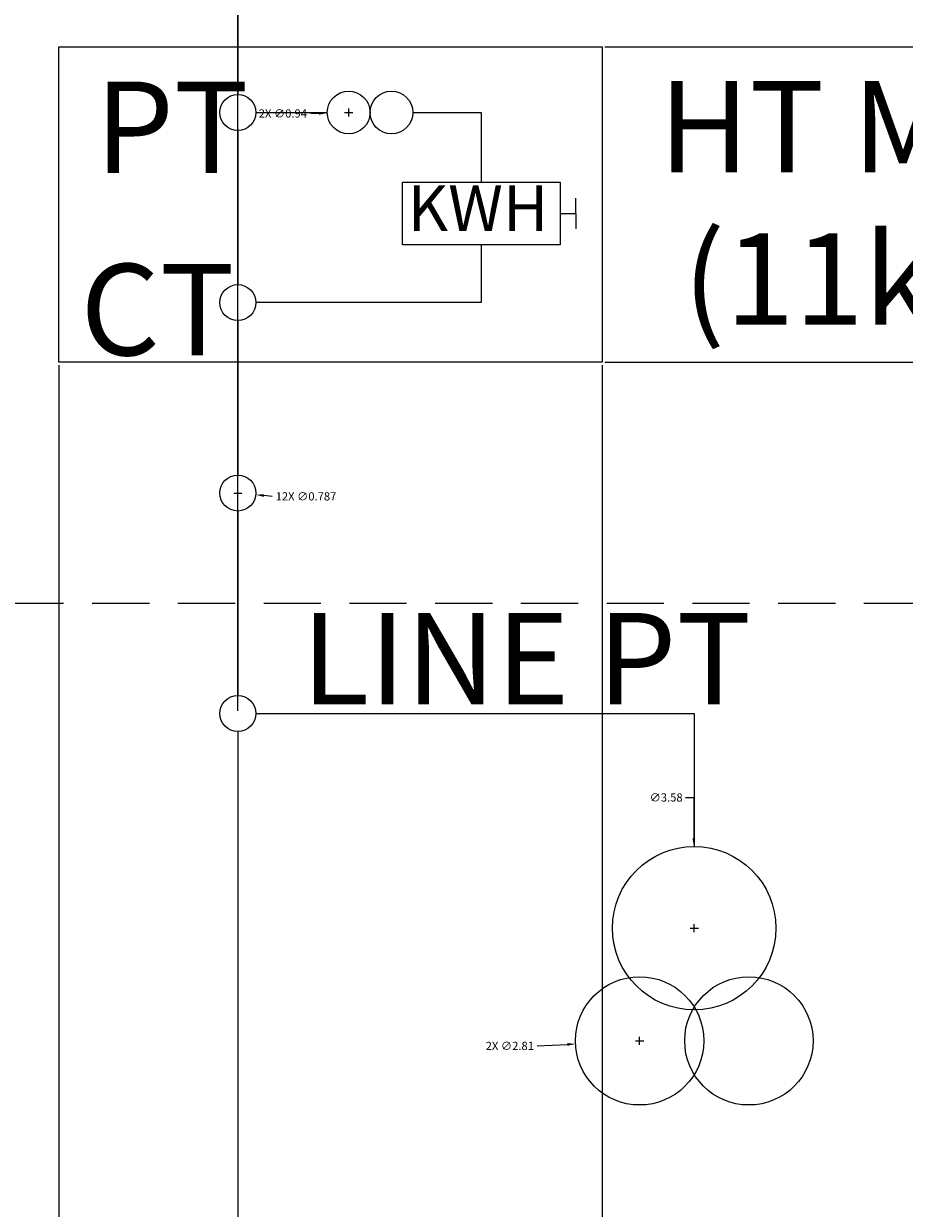
# Model space of a CAD drawing. Units: inches. Extents: x 412 to 584, y 208 to 437.
# Tile 25 of 28: x 495 to 514, y 387 to 413. Entities that reach past the tile are written whole.
import ezdxf

# ---------------------------------------------------------------- set-up
doc = ezdxf.new("R2010")
doc.units = ezdxf.units.IN
doc.header["$MEASUREMENT"] = 0
doc.linetypes.add('HIDDEN', pattern=[0.375, 0.25, -0.125])
for name, color, linetype, lineweight in [('A-ANNO-DIMS', 2, 'Continuous', 18), ('E-ANNO-TEXT', 7, 'Continuous', 18), ('E-ENCL', 8, 'Continuous', 18), ('E-ENCL-HIDN', 3, 'HIDDEN', 18), ('E-POWR-EQPM', 3, 'Continuous', 25)]:
    doc.layers.add(name, color=color, linetype=linetype, lineweight=lineweight)
doc.styles.get("Standard").update_dxf_attribs({"font": 'arial.ttf'})
doc.dimstyles.get("Standard").update_dxf_attribs({"dimtxt": 0.18, "dimasz": 0.18, "dimexe": 0.18, "dimexo": 0.0625, "dimgap": 0.09, "dimtad": 0, "dimtih": 1, "dimtoh": 1, "dimdec": 4, "dimzin": 0, "dimdsep": 46, "dimtxsty": 'Standard', "dimcen": 0.09, "dimadec": 0, "dimazin": 0, "dimtfac": 1, "dimtdec": 4, "dimtofl": 0, "dimtmove": 0, "dimatfit": 3, "dimfxl": 1, "dimtolj": 1, "dimtzin": 0, "dimarcsym": 0})

# ---------------------------------------------------------------- blocks, each defined once
blk = doc.blocks.new('*D17')
at = {"layer": 'A-ANNO-DIMS', "color": 0, "lineweight": -2, "transparency": 16777216}
for p, q in [((497.715, 426.185), (583.674, 426.185)), ((583.494, 426.005), (583.494, 323.031)), ((583.494, 219.693), (583.494, 322.667)), ((550.198, 219.513), (583.674, 219.513))]:
    blk.add_line(p, q, dxfattribs=at)
at = {"layer": 'A-ANNO-DIMS', "color": 0, "transparency": 16777216}
for points in [[(583.464, 426.005), (583.524, 426.005), (583.494, 426.185)], [(583.464, 219.693), (583.524, 219.693), (583.494, 219.513)]]:
    blk.add_solid(points, dxfattribs=at)
at = {"layer": 'Defpoints', "color": 0, "transparency": 16777216}
for p in [(497.652, 426.185), (550.135, 219.513), (583.494, 219.513)]:
    blk.add_point(p, dxfattribs=at)
at = {"layer": 'A-ANNO-DIMS', "color": 0, "transparency": 16777216, "insert": (583.494, 322.849), "char_height": 0.18, "attachment_point": 5}
blk.add_mtext('\\A1;206.67', dxfattribs=at)
blk = doc.blocks.new('*D20')
at = {"layer": 'A-ANNO-DIMS', "color": 0, "lineweight": -2, "transparency": 16777216}
for p, q in [((507.316, 412.35), (583.674, 412.35)), ((583.494, 412.17), (583.494, 406.444)), ((583.494, 400.355), (583.494, 406.08)), ((538.681, 400.175), (583.674, 400.175))]:
    blk.add_line(p, q, dxfattribs=at)
at = {"layer": 'A-ANNO-DIMS', "color": 0, "transparency": 16777216}
for points in [[(583.464, 412.17), (583.524, 412.17), (583.494, 412.35)], [(583.464, 400.355), (583.524, 400.355), (583.494, 400.175)]]:
    blk.add_solid(points, dxfattribs=at)
at = {"layer": 'Defpoints', "color": 0, "transparency": 16777216}
for p in [(507.254, 412.35), (538.619, 400.175), (583.494, 400.175)]:
    blk.add_point(p, dxfattribs=at)
at = {"layer": 'A-ANNO-DIMS', "color": 0, "transparency": 16777216, "insert": (583.494, 406.262), "char_height": 0.18, "attachment_point": 5}
blk.add_mtext('\\A1;12.175', dxfattribs=at)
blk = doc.blocks.new('*D21')
at = {"layer": 'A-ANNO-DIMS', "color": 0, "lineweight": -2, "transparency": 16777216}
for p, q in [((466.104, 400.237), (466.104, 437.465)), ((538.619, 400.237), (538.619, 437.465)), ((466.284, 437.285), (501.986, 437.285)), ((538.439, 437.285), (502.737, 437.285))]:
    blk.add_line(p, q, dxfattribs=at)
at = {"layer": 'A-ANNO-DIMS', "color": 0, "transparency": 16777216}
for points in [[(466.284, 437.315), (466.284, 437.255), (466.104, 437.285)], [(538.439, 437.315), (538.439, 437.255), (538.619, 437.285)]]:
    blk.add_solid(points, dxfattribs=at)
at = {"layer": 'Defpoints', "color": 0, "transparency": 16777216}
for p in [(538.619, 437.285), (466.104, 400.175), (538.619, 400.175)]:
    blk.add_point(p, dxfattribs=at)
at = {"layer": 'A-ANNO-DIMS', "color": 0, "transparency": 16777216, "insert": (502.361, 437.285), "char_height": 0.18, "attachment_point": 5}
blk.add_mtext('\\A1;72.51', dxfattribs=at)
blk = doc.blocks.new('*D27')
at = {"layer": 'A-ANNO-DIMS', "color": 0, "lineweight": -2, "transparency": 16777216}
for p, q in [((466.104, 400.237), (466.104, 437.465)), ((499.288, 397.825), (499.288, 437.465)), ((466.284, 437.285), (482.233, 437.285)), ((499.108, 437.285), (483.159, 437.285))]:
    blk.add_line(p, q, dxfattribs=at)
at = {"layer": 'A-ANNO-DIMS', "color": 0, "transparency": 16777216}
for points in [[(466.284, 437.315), (466.284, 437.255), (466.104, 437.285)], [(499.108, 437.315), (499.108, 437.255), (499.288, 437.285)]]:
    blk.add_solid(points, dxfattribs=at)
at = {"layer": 'Defpoints', "color": 0, "transparency": 16777216}
for p in [(499.288, 437.285), (466.104, 400.175), (499.288, 397.763)]:
    blk.add_point(p, dxfattribs=at)
at = {"layer": 'A-ANNO-DIMS', "color": 0, "transparency": 16777216, "insert": (482.696, 437.285), "char_height": 0.18, "attachment_point": 5}
blk.add_mtext('\\A1;33.184', dxfattribs=at)
blk = doc.blocks.new('*D28')
at = {"layer": 'A-ANNO-DIMS', "color": 0, "lineweight": -2, "transparency": 16777216}
for p, q in [((450.562, 256.635), (450.562, 437.465)), ((555.796, 256.635), (555.796, 437.465)), ((450.742, 437.285), (502.724, 437.285)), ((555.616, 437.285), (503.634, 437.285))]:
    blk.add_line(p, q, dxfattribs=at)
at = {"layer": 'A-ANNO-DIMS', "color": 0, "transparency": 16777216}
for points in [[(450.742, 437.315), (450.742, 437.255), (450.562, 437.285)], [(555.616, 437.315), (555.616, 437.255), (555.796, 437.285)]]:
    blk.add_solid(points, dxfattribs=at)
at = {"layer": 'Defpoints', "color": 0, "transparency": 16777216}
for p in [(555.796, 437.285), (450.562, 256.573), (555.796, 256.573)]:
    blk.add_point(p, dxfattribs=at)
at = {"layer": 'A-ANNO-DIMS', "color": 0, "transparency": 16777216, "insert": (503.179, 437.285), "char_height": 0.18, "attachment_point": 5}
blk.add_mtext('\\A1;105.23', dxfattribs=at)
blk = doc.blocks.new('*D31')
at = {"layer": 'A-ANNO-DIMS', "color": 0, "lineweight": -2, "transparency": 16777216}
for p, q in [((495.375, 405.385), (495.375, 208.233)), ((507.254, 405.385), (507.254, 208.233)), ((495.555, 208.413), (500.929, 208.413)), ((507.074, 208.413), (501.7, 208.413))]:
    blk.add_line(p, q, dxfattribs=at)
at = {"layer": 'A-ANNO-DIMS', "color": 0, "transparency": 16777216}
for points in [[(495.555, 208.443), (495.555, 208.383), (495.375, 208.413)], [(507.074, 208.443), (507.074, 208.383), (507.254, 208.413)]]:
    blk.add_solid(points, dxfattribs=at)
at = {"layer": 'Defpoints', "color": 0, "transparency": 16777216}
for p in [(495.375, 405.448), (507.254, 405.448), (507.254, 208.413)]:
    blk.add_point(p, dxfattribs=at)
at = {"layer": 'A-ANNO-DIMS', "color": 0, "transparency": 16777216, "insert": (501.314, 208.413), "char_height": 0.18, "attachment_point": 5}
blk.add_mtext('\\A1;11.88', dxfattribs=at)
blk = doc.blocks.new('*D32')
at = {"layer": 'A-ANNO-DIMS', "color": 0, "lineweight": -2, "transparency": 16777216}
for p, q in [((507.316, 412.35), (583.674, 412.35)), ((583.494, 412.17), (583.494, 409.081)), ((583.494, 405.628), (583.494, 408.717)), ((507.316, 405.448), (583.674, 405.448))]:
    blk.add_line(p, q, dxfattribs=at)
at = {"layer": 'A-ANNO-DIMS', "color": 0, "transparency": 16777216}
for points in [[(583.464, 412.17), (583.524, 412.17), (583.494, 412.35)], [(583.464, 405.628), (583.524, 405.628), (583.494, 405.448)]]:
    blk.add_solid(points, dxfattribs=at)
at = {"layer": 'Defpoints', "color": 0, "transparency": 16777216}
for p in [(507.254, 412.35), (507.254, 405.448), (583.494, 405.448)]:
    blk.add_point(p, dxfattribs=at)
at = {"layer": 'A-ANNO-DIMS', "color": 0, "transparency": 16777216, "insert": (583.494, 408.899), "char_height": 0.18, "attachment_point": 5}
blk.add_mtext('\\A1;6.902', dxfattribs=at)
blk = doc.blocks.new('*D46')
at = {"layer": 'A-ANNO-DIMS', "color": 0, "lineweight": -2, "transparency": 16777216}
for p, q in [((509.075, 395.927), (509.255, 395.927)), ((509.255, 395.927), (509.259, 395.034)), ((509.267, 392.977), (509.267, 393.157)), ((509.177, 393.067), (509.357, 393.067))]:
    blk.add_line(p, q, dxfattribs=at)
at = {"layer": 'A-ANNO-DIMS', "color": 0, "transparency": 16777216}
blk.add_solid([(509.289, 395.035), (509.229, 395.034), (509.26, 394.854)], dxfattribs=at)
at = {"layer": 'Defpoints', "color": 0, "transparency": 16777216}
for p in [(509.26, 394.854), (509.275, 391.279)]:
    blk.add_point(p, dxfattribs=at)
at = {"layer": 'A-ANNO-DIMS', "color": 0, "transparency": 16777216, "insert": (508.653, 395.927), "char_height": 0.18, "attachment_point": 5}
blk.add_mtext('\\A1;∅3.58', dxfattribs=at)
blk = doc.blocks.new('*D47')
at = {"layer": 'A-ANNO-DIMS', "color": 0, "lineweight": -2, "transparency": 16777216}
for p, q in [((507.982, 390.602), (508.162, 390.602)), ((508.072, 390.512), (508.072, 390.692)), ((505.83, 390.492), (506.491, 390.525))]:
    blk.add_line(p, q, dxfattribs=at)
at = {"layer": 'A-ANNO-DIMS', "color": 0, "transparency": 16777216}
blk.add_solid([(506.49, 390.555), (506.493, 390.495), (506.671, 390.533)], dxfattribs=at)
at = {"layer": 'Defpoints', "color": 0, "transparency": 16777216}
for p in [(509.474, 390.671), (506.671, 390.533)]:
    blk.add_point(p, dxfattribs=at)
at = {"layer": 'A-ANNO-DIMS', "color": 0, "transparency": 16777216, "insert": (505.235, 390.492), "char_height": 0.18, "attachment_point": 5}
blk.add_mtext('\\A1;2X ∅2.81', dxfattribs=at)
blk = doc.blocks.new('*D48')
at = {"layer": 'A-ANNO-DIMS', "color": 0, "lineweight": -2, "transparency": 16777216}
for p, q in [((499.198, 402.587), (499.378, 402.587)), ((499.288, 402.497), (499.288, 402.677)), ((500.038, 402.514), (499.859, 402.532))]:
    blk.add_line(p, q, dxfattribs=at)
at = {"layer": 'A-ANNO-DIMS', "color": 0, "transparency": 16777216}
blk.add_solid([(499.861, 402.561), (499.856, 402.502), (499.679, 402.549)], dxfattribs=at)
at = {"layer": 'Defpoints', "color": 0, "transparency": 16777216}
for p in [(498.896, 402.625), (499.679, 402.549)]:
    blk.add_point(p, dxfattribs=at)
at = {"layer": 'A-ANNO-DIMS', "color": 0, "transparency": 16777216, "insert": (500.779, 402.514), "char_height": 0.18, "attachment_point": 5}
blk.add_mtext('\\A1;12X ∅0.787', dxfattribs=at)
blk = doc.blocks.new('*D50')
at = {"layer": 'A-ANNO-DIMS', "color": 0, "lineweight": -2, "transparency": 16777216}
for p, q in [((500.884, 410.891), (501.064, 410.895)), ((501.622, 410.912), (501.802, 410.912)), ((501.712, 410.822), (501.712, 411.002))]:
    blk.add_line(p, q, dxfattribs=at)
at = {"layer": 'A-ANNO-DIMS', "color": 0, "transparency": 16777216}
blk.add_solid([(501.063, 410.925), (501.065, 410.865), (501.244, 410.9)], dxfattribs=at)
at = {"layer": 'Defpoints', "color": 0, "transparency": 16777216}
for p in [(501.244, 410.9), (502.179, 410.925)]:
    blk.add_point(p, dxfattribs=at)
at = {"layer": 'A-ANNO-DIMS', "color": 0, "transparency": 16777216, "insert": (500.273, 410.891), "char_height": 0.18, "attachment_point": 5}
blk.add_mtext('\\A1;2X ∅0.94', dxfattribs=at)

msp = doc.modelspace()

# ---------------------------------------------------------------- linework, layer by layer
at = {"layer": 'E-ENCL'}
msp.add_lwpolyline([(495.3746, 412.3496), (507.2538, 412.3496), (507.2538, 405.448), (495.3746, 405.448)], close=True, dxfattribs=at)
at = {"layer": 'E-ENCL-HIDN', "ltscale": 5}
msp.add_lwpolyline([(466.1037, 400.175), (538.6186, 400.175), (538.6186, 360.1961), (466.1037, 360.1961)], close=True, dxfattribs=at)
at = {"layer": 'E-POWR-EQPM'}
for p, q in [((499.2878, 414.6932), (499.2878, 411.7856)), ((499.2878, 411.7856), (499.2878, 411.3059)), ((499.6813, 410.9124), (501.2439, 410.9124)), ((503.1145, 410.9124), (504.6111, 410.9124)), ((504.6111, 410.9124), (504.6111, 409.3893)), ((499.2878, 410.519), (499.2878, 407.1463)), ((506.6779, 408.7039), (506.6779, 409.0373)), ((506.3363, 408.7039), (506.6779, 408.7039)), ((506.6779, 408.7039), (506.6779, 408.3705)), ((504.6111, 408.0186), (504.6111, 406.7528)), ((504.6111, 406.7528), (499.6813, 406.7528)), ((499.2878, 406.3594), (499.2878, 402.9807)), ((499.2878, 402.1938), (499.2878, 398.1561)), ((499.6813, 397.7626), (509.2671, 397.7626)), ((509.2671, 397.7626), (509.2671, 394.8544)), ((499.2878, 397.3692), (499.2878, 385.9599))]:
    msp.add_line(p, q, dxfattribs=at)
msp.add_lwpolyline([(502.8859, 409.3893), (506.3363, 409.3893), (506.3363, 408.0186), (502.8859, 408.0186)], close=True, dxfattribs=at)
for centre, radius in [((499.2878, 410.9124), 0.3935), ((501.7115, 410.9124), 0.4677), ((502.6469, 410.9124), 0.4677), ((499.2878, 406.7528), 0.3935), ((499.2878, 402.5873), 0.3935), ((499.2878, 397.7626), 0.3935), ((509.2671, 393.0667), 1.7877), ((508.0725, 390.6024), 1.4033), ((510.4617, 390.6024), 1.4033)]:
    msp.add_circle(centre, radius, dxfattribs=at)

# ---------------------------------------------------------------- texts
at = {"layer": 'E-ANNO-TEXT', "attachment_point": 1}
for s, width, heights, insert, char_height in [('\\pxqc;PT', 13.633448, [2.9648], (491.0285, 411.5901), 2), ('\\pxqc;HT Metering\\P(11kV, REB)', 20.444042, [7.5463], (506.0251, 411.601), 2), ('\\pxqc;KWH', 13.633448, [2.9648], (497.7238, 409.321), 1), ('\\pxqc;CT', 13.633448, [2.9648], (490.7153, 407.5997), 2), ('\\pxqc;LINE PT', 13.633448, [2.9648], (498.7777, 399.9631), 2)]:
    msp.add_mtext_dynamic_manual_height_columns(s, width=width, gutter_width=1, heights=heights, dxfattribs=dict(at, insert=insert, char_height=char_height))

# ---------------------------------------------------------------- dimensions: what is measured, and where the dimension line sits
at = {"layer": 'A-ANNO-DIMS'}
for base, p1, p2, override, picture, middle in [((555.7959, 437.2847), (450.562, 256.5729), (555.7959, 256.5729), {"dimdec": 2, "dimlfac": 1, "dimrnd": 0, "dimzin": 0, "dimdsep": 46, "dimlunit": 2}, '*D28', (503.1789, 437.2847)), ((538.6186, 437.2847), (466.1037, 400.175), (538.6186, 400.175), {"dimdec": 2, "dimlfac": 1, "dimrnd": 0, "dimzin": 0, "dimdsep": 46, "dimlunit": 2}, '*D21', (502.3612, 437.2847)), ((499.2878, 437.2847), (466.1037, 400.175), (499.2878, 397.7626), {"dimdec": 3, "dimlfac": 1, "dimrnd": 0, "dimzin": 0, "dimdsep": 46, "dimlunit": 2}, '*D27', (482.6958, 437.2847)), ((507.2538, 208.4133), (495.3746, 405.448), (507.2538, 405.448), {"dimdec": 2, "dimlfac": 1, "dimrnd": 0, "dimzin": 0, "dimdsep": 46, "dimlunit": 2}, '*D31', (501.3142, 208.4133))]:
    dim = msp.add_linear_dim(base=base, p1=p1, p2=p2, dimstyle='Standard', override=override, dxfattribs=at)
    dim.commit()
    dim.dimension.update_dxf_attribs({"geometry": picture, "text_midpoint": middle})
for base, p1, p2, override, picture, middle in [((583.4937, 219.5133), (497.6523, 426.1847), (550.1351, 219.5133), {"dimdec": 2, "dimlfac": 1, "dimrnd": 0, "dimzin": 0, "dimdsep": 46, "dimlunit": 2}, '*D17', (583.4937, 322.849)), ((583.4937, 400.175), (507.2538, 412.3496), (538.6186, 400.175), {"dimdec": 3, "dimlfac": 1, "dimrnd": 0, "dimzin": 0, "dimdsep": 46, "dimlunit": 2}, '*D20', (583.4937, 406.2623)), ((583.4937, 405.448), (507.2538, 412.3496), (507.2538, 405.448), {"dimdec": 3, "dimlfac": 1, "dimrnd": 0, "dimzin": 0, "dimdsep": 46, "dimlunit": 2}, '*D32', (583.4937, 408.8988))]:
    dim = msp.add_linear_dim(base=base, p1=p1, p2=p2, angle=90, dimstyle='Standard', override=override, dxfattribs=at)
    dim.commit()
    dim.dimension.update_dxf_attribs({"geometry": picture, "text_midpoint": middle})
for p1, p2, text, override, picture, middle in [((502.179, 410.9247), (501.244, 410.9001), '2X <>', {"dimdec": 2, "dimlfac": 1, "dimrnd": 0, "dimzin": 0, "dimdsep": 46, "dimlunit": 2}, '*D50', (500.8841, 410.8906)), ((498.8962, 402.6254), (499.6794, 402.5491), '12X <>', {"dimdec": 3, "dimlfac": 1, "dimrnd": 0, "dimzin": 0, "dimdsep": 46, "dimlunit": 2}, '*D48', (500.0377, 402.5142)), ((509.4741, 390.6713), (506.6709, 390.5335), '2X <>', {"dimdec": 2, "dimlfac": 1, "dimrnd": 0, "dimzin": 0, "dimdsep": 46, "dimlunit": 2}, '*D47', (505.83, 390.4921))]:
    dim = msp.add_diameter_dim_2p(p1=p1, p2=p2, text=text, dimstyle='Standard', override=override, dxfattribs=at)
    dim.commit()
    dim.dimension.update_dxf_attribs({"geometry": picture, "text_midpoint": middle, "dimtype": 163})
dim = msp.add_diameter_dim_2p(p1=(509.2746, 391.2789), p2=(509.2596, 394.8544), dimstyle='Standard', override={"dimdec": 2, "dimlfac": 1, "dimrnd": 0, "dimzin": 0, "dimdsep": 46, "dimlunit": 2}, dxfattribs=at)
dim.commit()
dim.dimension.update_dxf_attribs({"geometry": '*D46', "text_midpoint": (508.6532, 395.9271), "dimtype": 163})

doc.saveas('drawing.dxf')
